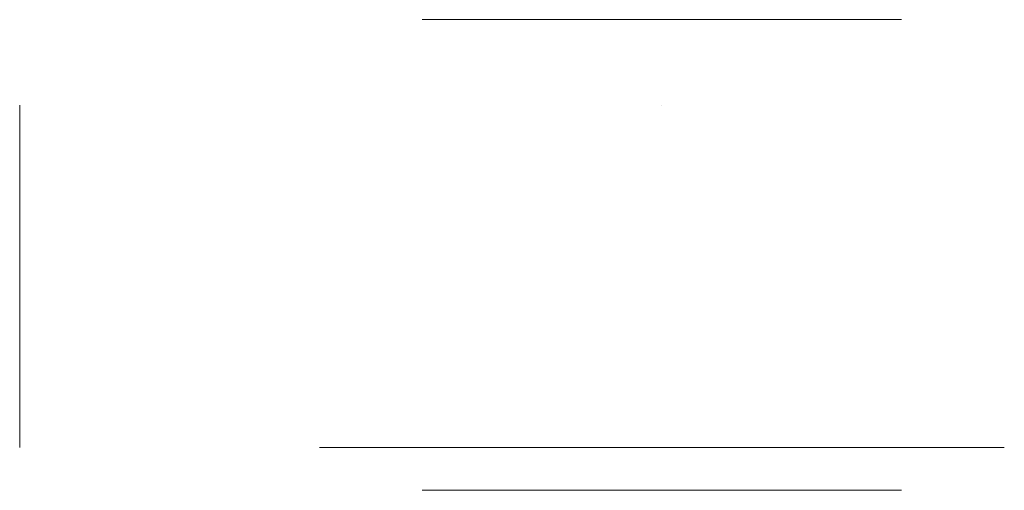
# Model space of a CAD drawing. Units: millimetres. Extents: x 0 to 115, y -188 to -133.
import ezdxf

# ---------------------------------------------------------------- set-up
doc = ezdxf.new("R2010")
doc.units = ezdxf.units.MM
doc.layers.add('M-CONS', color=8, linetype='Continuous', lineweight=13)

msp = doc.modelspace()

# ---------------------------------------------------------------- linework, layer by layer
at = {"layer": 'M-CONS', "extrusion": (-1, 0, 0)}
for p, q in [((0, -163.26, -22.43), (0, -143.26, -22.43)), ((0, -143.26, -22.43), (0, -143.26, -14.03)), ((0, -163.26, 22.57), (0, -159.26, 22.57)), ((0, -159.26, 22.57), (0, -159.26, 18.98)), ((0, -163.26, 22.57), (0, -167.26, 22.57)), ((0, -183.26, -22.43), (0, -163.26, -22.43)), ((0, -167.26, 18.98), (0, -167.26, 22.57)), ((0, -183.26, -14.03), (0, -183.26, -22.43))]:
    msp.add_line(p, q, dxfattribs=at)
at = {"layer": 'M-CONS', "extrusion": (0, -1, 0)}
msp.add_line((75, -143.26, -31.53), (75, -143.26, -31.53), dxfattribs=at)
at = {"layer": 'M-CONS', "extrusion": (-1, 0, 0)}
msp.add_lwpolyline([(143.26, 44.16), (183.26, 44.16), (183.26, 25.16, 0.420204), (143.26, 25.16), (143.26, 44.16), (143.26, 25.16)], format="xyb", dxfattribs=at)
at = {"layer": 'M-CONS', "extrusion": (0, -1, 0)}
for centre, radius in [((75, 8.47, 133.26), 28), ((75, 8.47, 183.26), 40), ((75, 8.47, 188.26), 28)]:
    msp.add_circle(centre, radius, dxfattribs=at)
at = {"layer": 'M-CONS', "extrusion": (-1, 0, 0)}
for radius, start, end in [(28, 44.4153, 135.5847), (28, 224.4153, 315.5847), (14, 106.6015, 73.3985)]:
    msp.add_arc((163.26, 5.57), radius, start, end, dxfattribs=at)

doc.saveas('drawing.dxf')
